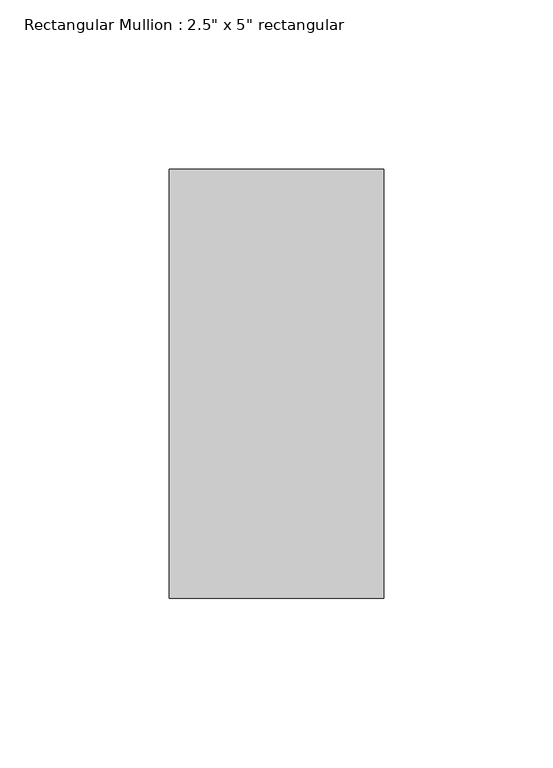
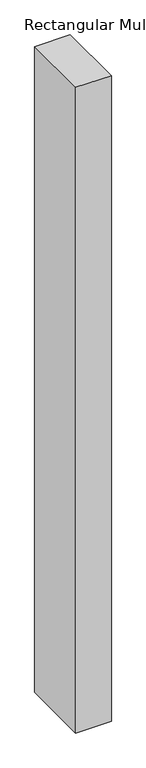
"""IFC4 building model written with IfcOpenShell, lengths in millimetres: member geometry."""

from ifc_helpers import new_model, si_unit, frame, origin, place, context, project, spatial, polyline, outline, extrude, source, transform, mapped, element, save


def member_3d117b0e(model_context):
    return source(origin(), model_context, "Body", "SweptSolid", [
        extrude(outline(polyline([(0.0, 63.5), (0.0, -63.5), (-63.5, -63.5), (-63.5, 63.5), (0.0, 63.5)])), frame((0.0, 0.0, -1219.1999999), z_axis=(0.0, 0.0, 1.0), x_axis=(1.0, 0.0, 0.0)), (0.0, 0.0, 1.0), 1219.1999999),
    ])


if __name__ == "__main__":
    model = new_model("IFC4")
    model_context = context("Model", 3, world=origin())
    ifc_project = project(units=[si_unit("LENGTHUNIT", "METRE", prefix="MILLI")], contexts=[model_context])
    site = spatial("IfcSite", under=ifc_project)
    building = spatial("IfcBuilding", under=site)
    placement = place(None, origin())
    member_shape = member_3d117b0e(model_context)
    element("IfcMember", 1, ObjectType="Rectangular Mullion : 2.5\" x 5\" rectangular", at=placement, inside=building, context=model_context, shape_type="MappedRepresentation", body=[
        mapped(member_shape, transform((0.0, 0.0, 0.0), x_axis=(1.0, 0.0, 0.0), y_axis=(0.0, 1.0, 0.0), z_axis=(0.0, 0.0, 1.0))),
    ])
    save(model, "model.ifc")

# Revit data of these elements
# Type "Rectangular Mullion : 2.5\" x 5\" rectangular"
#   built-in parameter 1007304 = 0.416667 (stored number, unit not read)
#   built-in parameter 1007301 = 0.104167 (stored number, unit not read)
#   built-in parameter 1007300 = 0.104167 (stored number, unit not read)
# Element 1 (IfcMember, "Rectangular Mullion : 2.5\" x 5\" rectangular")
#   Materials on its faces: "Aluminum"
# Materials
#   "Aluminum": class "Metal", colour RGB 247 247 247, transparency 0, Description = "Aluminum 6061", Cost = 0
